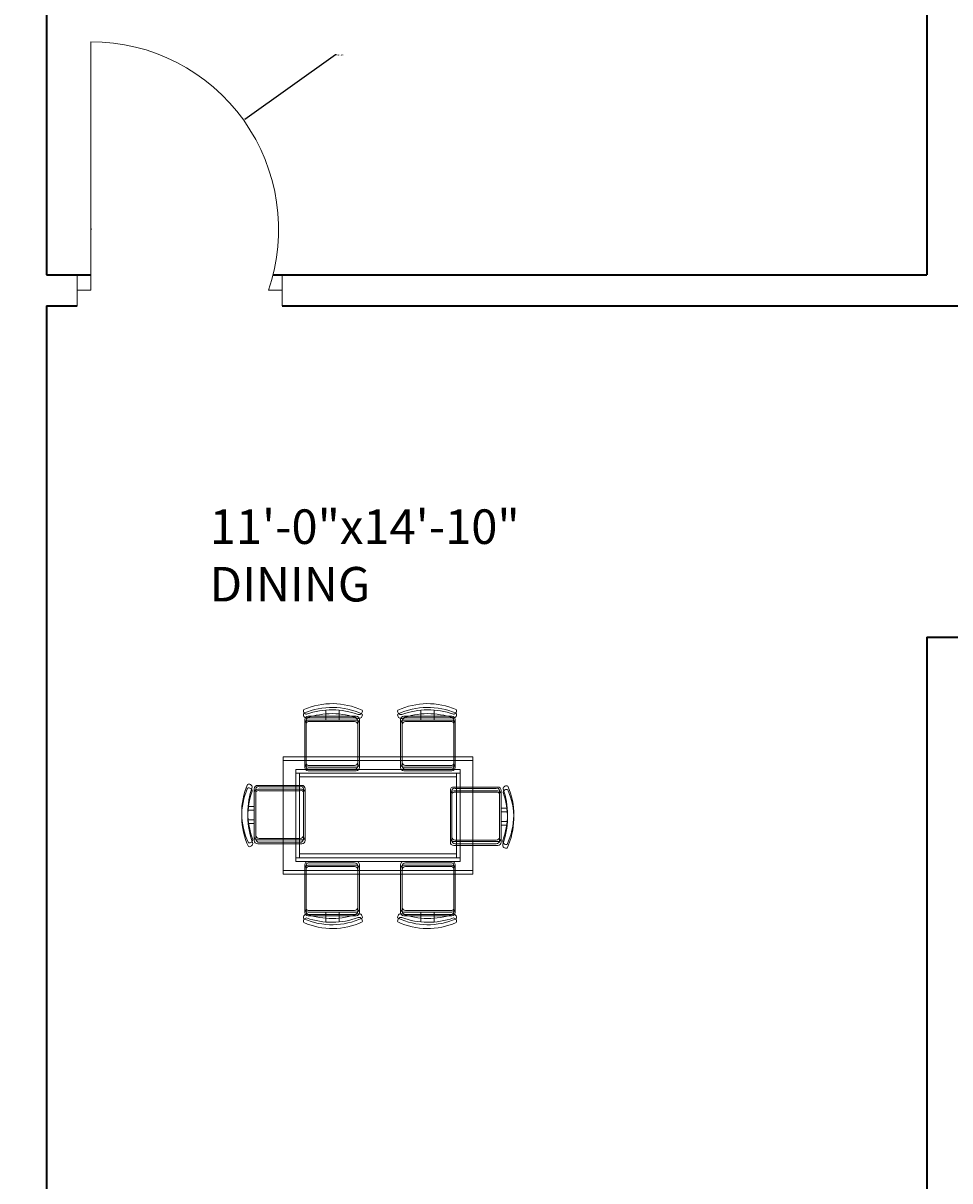
# Model space of a CAD drawing. Units: inches. Extents: x 2163 to 2982, y 1024 to 2288.
# Tile 20 of 22: x 2583 to 2718, y 1885 to 2053. Entities that reach past the tile are written whole.
import ezdxf

# ---------------------------------------------------------------- set-up
doc = ezdxf.new("R2010")
doc.units = ezdxf.units.IN
for name, color, linetype, lineweight in [('A-ANNO-DIMS', 2, 'Continuous', 18), ('A-AREA-IDEN', 7, 'Continuous', 18), ('A-DOOR', 11, 'Continuous', 18), ('A-FURN', 8, 'Continuous', 13), ('A-WALL', 7, 'Continuous', 35)]:
    doc.layers.add(name, color=color, linetype=linetype, lineweight=lineweight)
doc.styles.get("Standard").update_dxf_attribs({"font": 'arial.ttf'})
doc.dimstyles.get("Standard").update_dxf_attribs({"dimtxt": 0.18, "dimasz": 0.18, "dimexe": 0.18, "dimexo": 0.0625, "dimgap": 0.09, "dimtad": 0, "dimtih": 1, "dimtoh": 1, "dimdec": 4, "dimzin": 0, "dimdsep": 46, "dimtxsty": 'Standard', "dimcen": 0.09, "dimadec": 0, "dimazin": 0, "dimtfac": 1, "dimtdec": 4, "dimtofl": 0, "dimtmove": 0, "dimatfit": 3, "dimfxl": 1, "dimtolj": 1, "dimtzin": 0, "dimarcsym": 0})

# ---------------------------------------------------------------- blocks, each defined once
blk = doc.blocks.new('TABLE-DINING')
for points in [[(0, 17.02), (27.45, 17.02), (27.45, 0.55), (0, 0.55)], [(0, 17.02), (27.45, 17.02), (27.45, 0.55), (0, 0.55)], [(0, 17.02), (27.45, 17.02), (27.45, 0.55), (0, 0.55)], [(0, 17.02), (27.45, 17.02), (27.45, 0.55), (0, 0.55)], [(0, 16.47), (27.45, 16.47), (27.45, 0), (0, 0)], [(0, 16.47), (27.45, 16.47), (27.45, 0), (0, 0)], [(0, 16.47), (27.45, 16.47), (27.45, 0), (0, 0)], [(0, 16.47), (27.45, 16.47), (27.45, 0), (0, 0)], [(1.83, 15.19), (25.62, 15.19), (25.62, 2.38), (1.83, 2.38)], [(1.83, 15.19), (25.62, 15.19), (25.62, 2.38), (1.83, 2.38)], [(1.83, 15.19), (25.62, 15.19), (25.62, 2.38), (1.83, 2.38)], [(1.83, 15.19), (25.62, 15.19), (25.62, 2.38), (1.83, 2.38)], [(1.83, 14.64), (25.62, 14.64), (25.62, 1.83), (1.83, 1.83)], [(1.83, 14.64), (25.62, 14.64), (25.62, 1.83), (1.83, 1.83)], [(1.83, 14.64), (25.62, 14.64), (25.62, 1.83), (1.83, 1.83)], [(1.83, 14.64), (25.62, 14.64), (25.62, 1.83), (1.83, 1.83)], [(2.38, 14.64), (25.07, 14.64), (25.07, 2.93), (2.38, 2.93)], [(2.38, 14.64), (25.07, 14.64), (25.07, 2.93), (2.38, 2.93)], [(2.38, 14.64), (25.07, 14.64), (25.07, 2.93), (2.38, 2.93)], [(2.38, 14.64), (25.07, 14.64), (25.07, 2.93), (2.38, 2.93)], [(2.38, 14.09), (25.07, 14.09), (25.07, 2.38), (2.38, 2.38)], [(2.38, 14.09), (25.07, 14.09), (25.07, 2.38), (2.38, 2.38)], [(2.38, 14.09), (25.07, 14.09), (25.07, 2.38), (2.38, 2.38)], [(2.38, 14.09), (25.07, 14.09), (25.07, 2.38), (2.38, 2.38)]]:
    blk.add_lwpolyline(points, close=True)
blk = doc.blocks.new('*D29')
at = {"layer": 'A-ANNO-DIMS', "color": 0, "lineweight": -2, "transparency": 16777216}
for p, q in [((2285.34, 1738.83), (2285.34, 2288.1)), ((2285.52, 2287.92), (2576.05, 2287.92)), ((2867.16, 2287.92), (2576.63, 2287.92)), ((2867.34, 2229.33), (2867.34, 2288.1))]:
    blk.add_line(p, q, dxfattribs=at)
at = {"layer": 'A-ANNO-DIMS', "color": 0, "transparency": 16777216}
for points in [[(2285.52, 2287.95), (2285.52, 2287.89), (2285.34, 2287.92)], [(2867.16, 2287.95), (2867.16, 2287.89), (2867.34, 2287.92)]]:
    blk.add_solid(points, dxfattribs=at)
at = {"layer": 'Defpoints', "color": 0, "transparency": 16777216}
for p in [(2867.34, 2287.92), (2867.34, 2229.27), (2285.34, 1738.77)]:
    blk.add_point(p, dxfattribs=at)
at = {"layer": 'A-ANNO-DIMS', "color": 0, "transparency": 16777216, "insert": (2576.34, 2287.92), "char_height": 0.18, "attachment_point": 5}
blk.add_mtext('\\A1;582', dxfattribs=at)
blk = doc.blocks.new('*D47')
at = {"layer": 'A-ANNO-DIMS', "color": 0, "lineweight": -2, "transparency": 16777216}
for p, q in [((2628.67, 2048.1), (2615.54, 2038.74)), ((2628.85, 2048.1), (2628.67, 2048.1)), ((2593.2, 2022.85), (2593.38, 2022.85)), ((2593.29, 2022.76), (2593.29, 2022.94))]:
    blk.add_line(p, q, dxfattribs=at)
at = {"layer": 'A-ANNO-DIMS', "color": 0, "transparency": 16777216}
blk.add_solid([(2615.53, 2038.76), (2615.56, 2038.71), (2615.4, 2038.63)], dxfattribs=at)
at = {"layer": 'Defpoints', "color": 0, "transparency": 16777216}
for p in [(2615.4, 2038.63), (2593.29, 2022.85)]:
    blk.add_point(p, dxfattribs=at)
at = {"layer": 'A-ANNO-DIMS', "color": 0, "transparency": 16777216, "insert": (2629.4, 2048.1), "char_height": 0.18, "attachment_point": 5}
blk.add_mtext('\\A1;R27.165', dxfattribs=at)

msp = doc.modelspace()

# ---------------------------------------------------------------- linework, layer by layer
at = {"layer": 'A-DOOR'}
for p, q in [((2593.2852, 2014.0188), (2593.2852, 2050.0188)), ((2591.2852, 2016.2688), (2591.2852, 2011.7688)), ((2620.9736, 2016.2688), (2620.9736, 2011.7688)), ((2591.2852, 2011.7688), (2591.2852, 2014.0188)), ((2591.2852, 2014.0188), (2593.2852, 2014.0188)), ((2620.9736, 2014.0188), (2618.9736, 2014.0188)), ((2620.9736, 2011.7688), (2620.9736, 2014.0188))]:
    msp.add_line(p, q, dxfattribs=at)
msp.add_arc((2593.2852, 2022.8537), 27.1652, 341.020745, 90, dxfattribs=at)
at = {"layer": 'A-FURN'}
for points in [[(2624.5142, 1952.6105, -0.17580919), (2631.9896, 1952.5539, 0.57839206), (2632.556, 1953.1766, 0.21452438), (2624.1178, 1953.2899, 0.55201397), (2624.5142, 1952.6105, -0.06507904)], [(2624.5142, 1952.6105, -0.17580919), (2631.9896, 1952.5539, 0.57839206), (2632.556, 1953.1766, 0.21452438), (2624.1178, 1953.2899, 0.55201397), (2624.5142, 1952.6105, -0.06507904)], [(2624.5142, 1952.6103, -0.17580919), (2631.9896, 1952.5536, 0.57839206), (2632.556, 1953.1764, 0.21452438), (2624.1178, 1953.2896, 0.55201397), (2624.5142, 1952.6103, -0.06507904)], [(2624.5142, 1952.6103, -0.17580919), (2631.9896, 1952.5536, 0.57839206), (2632.556, 1953.1764, 0.21452438), (2624.1178, 1953.2896, 0.55201397), (2624.5142, 1952.6103, -0.06507904)], [(2624.5142, 1952.0616, -0.17580919), (2631.9896, 1952.005, 0.57839206), (2632.556, 1952.6277, 0.21452438), (2624.1178, 1952.741, 0.55201397), (2624.5142, 1952.0616, -0.06507904)], [(2624.5142, 1952.0616, -0.17580919), (2631.9896, 1952.005, 0.57839206), (2632.556, 1952.6277, 0.21452438), (2624.1178, 1952.741, 0.55201397), (2624.5142, 1952.0616, -0.06507904)], [(2624.5142, 1952.0613, -0.17580919), (2631.9896, 1952.0047, 0.57839206), (2632.556, 1952.6274, 0.21452438), (2624.1178, 1952.7407, 0.55201397), (2624.5142, 1952.0613, -0.06507904)], [(2624.5142, 1952.0613, -0.17580919), (2631.9896, 1952.0047, 0.57839206), (2632.556, 1952.6274, 0.21452438), (2624.1178, 1952.7407, 0.55201397), (2624.5142, 1952.0613, -0.06507904)], [(2638.283, 1952.5539, -0.57839206), (2637.7167, 1953.1766, -0.21452438), (2646.1548, 1953.2899, -0.55201397), (2645.7584, 1952.6105, 0.1758092), (2638.283, 1952.5539)], [(2638.283, 1952.5539, -0.57839206), (2637.7167, 1953.1766, -0.21452438), (2646.1548, 1953.2899, -0.55201397), (2645.7584, 1952.6105, 0.1758092), (2638.283, 1952.5539)], [(2638.283, 1952.5536, -0.57839206), (2637.7167, 1953.1764, -0.21452438), (2646.1549, 1953.2896, -0.55201397), (2645.7584, 1952.6103, 0.1758092), (2638.283, 1952.5536)], [(2638.283, 1952.5536, -0.57839206), (2637.7167, 1953.1764, -0.21452438), (2646.1549, 1953.2896, -0.55201397), (2645.7584, 1952.6103, 0.1758092), (2638.283, 1952.5536)], [(2638.283, 1952.005, -0.57839206), (2637.7167, 1952.6277, -0.21452438), (2646.1548, 1952.741, -0.55201397), (2645.7584, 1952.0616, 0.1758092), (2638.283, 1952.005)], [(2638.283, 1952.005, -0.57839206), (2637.7167, 1952.6277, -0.21452438), (2646.1548, 1952.741, -0.55201397), (2645.7584, 1952.0616, 0.1758092), (2638.283, 1952.005)], [(2638.283, 1952.0047, -0.57839206), (2637.7167, 1952.6274, -0.21452438), (2646.1549, 1952.7407, -0.55201397), (2645.7584, 1952.0613, 0.1758092), (2638.283, 1952.0047)], [(2638.283, 1952.0047, -0.57839206), (2637.7167, 1952.6274, -0.21452438), (2646.1549, 1952.7407, -0.55201397), (2645.7584, 1952.0613, 0.1758092), (2638.283, 1952.0047)], [(2631.6725, 1952.3105), (2624.7325, 1952.3105, 0.41421356), (2624.247, 1951.825), (2624.247, 1945.4438, 0.41421356), (2624.7325, 1944.9583), (2631.6725, 1944.9583, 0.41421356), (2632.158, 1945.4438), (2632.158, 1951.825, 0.41421356), (2631.6725, 1952.3105)], [(2631.6725, 1952.3105), (2624.7325, 1952.3105, 0.41421356), (2624.247, 1951.825), (2624.247, 1945.4438, 0.41421356), (2624.7325, 1944.9583), (2631.6725, 1944.9583, 0.41421356), (2632.158, 1945.4438), (2632.158, 1951.825, 0.41421356), (2631.6725, 1952.3105)], [(2631.6725, 1952.3102), (2624.7326, 1952.3102, 0.41421356), (2624.247, 1951.8247), (2624.247, 1945.4436, 0.41421356), (2624.7326, 1944.958), (2631.6725, 1944.958, 0.41421356), (2632.158, 1945.4436), (2632.158, 1951.8247, 0.41421356), (2631.6725, 1952.3102)], [(2631.6725, 1952.3102), (2624.7326, 1952.3102, 0.41421356), (2624.247, 1951.8247), (2624.247, 1945.4436, 0.41421356), (2624.7326, 1944.958), (2631.6725, 1944.958, 0.41421356), (2632.158, 1945.4436), (2632.158, 1951.8247, 0.41421356), (2631.6725, 1952.3102)], [(2629.2348, 1952.3105), (2629.2348, 1953.1882, -0.06475861)], [(2629.2348, 1952.3105), (2629.2348, 1953.1882, -0.06475861)], [(2629.2348, 1952.3102), (2629.2348, 1953.1879, -0.06475861)], [(2629.2348, 1952.3102), (2629.2348, 1953.1879, -0.06475861)], [(2629.2348, 1951.7616), (2629.2348, 1952.6393, -0.06475861)], [(2629.2348, 1951.7616), (2629.2348, 1952.6393, -0.06475861)], [(2629.2348, 1951.7613), (2629.2348, 1952.639, -0.06475861)], [(2629.2348, 1951.7613), (2629.2348, 1952.639, -0.06475861)], [(2645.5401, 1952.3105, -0.41421356), (2646.0256, 1951.825), (2646.0256, 1945.4438, -0.41421356), (2645.5401, 1944.9583), (2638.6001, 1944.9583, -0.41421356), (2638.1146, 1945.4438), (2638.1146, 1951.825, -0.41421356), (2638.6001, 1952.3105), (2645.5401, 1952.3105)], [(2645.5401, 1952.3105, -0.41421356), (2646.0256, 1951.825), (2646.0256, 1945.4438, -0.41421356), (2645.5401, 1944.9583), (2638.6001, 1944.9583, -0.41421356), (2638.1146, 1945.4438), (2638.1146, 1951.825, -0.41421356), (2638.6001, 1952.3105), (2645.5401, 1952.3105)], [(2645.5401, 1952.3102, -0.41421356), (2646.0256, 1951.8247), (2646.0256, 1945.4436, -0.41421356), (2645.5401, 1944.958), (2638.6002, 1944.958, -0.41421356), (2638.1146, 1945.4436), (2638.1146, 1951.8247, -0.41421356), (2638.6002, 1952.3102), (2645.5401, 1952.3102)], [(2645.5401, 1952.3102, -0.41421356), (2646.0256, 1951.8247), (2646.0256, 1945.4436, -0.41421356), (2645.5401, 1944.958), (2638.6002, 1944.958, -0.41421356), (2638.1146, 1945.4436), (2638.1146, 1951.8247, -0.41421356), (2638.6002, 1952.3102), (2645.5401, 1952.3102)], [(2641.0378, 1952.3105), (2641.0378, 1953.1882, 0.06475861)], [(2641.0378, 1952.3105), (2641.0378, 1953.1882, 0.06475861)], [(2641.0378, 1952.3102), (2641.0378, 1953.1879, 0.06475861)], [(2641.0378, 1952.3102), (2641.0378, 1953.1879, 0.06475861)], [(2641.0378, 1951.7616), (2641.0378, 1952.6393, 0.06475861)], [(2641.0378, 1951.7616), (2641.0378, 1952.6393, 0.06475861)], [(2641.0378, 1951.7613), (2641.0378, 1952.639, 0.06475861)], [(2641.0378, 1951.7613), (2641.0378, 1952.639, 0.06475861)], [(2631.6725, 1951.7616), (2624.7325, 1951.7616, 0.41421356), (2624.247, 1951.2761), (2624.247, 1944.8949, 0.41421356), (2624.7325, 1944.4094), (2631.6725, 1944.4094, 0.41421356), (2632.158, 1944.8949), (2632.158, 1951.2761, 0.41421356), (2631.6725, 1951.7616)], [(2631.6725, 1951.7616), (2624.7325, 1951.7616, 0.41421356), (2624.247, 1951.2761), (2624.247, 1944.8949, 0.41421356), (2624.7325, 1944.4094), (2631.6725, 1944.4094, 0.41421356), (2632.158, 1944.8949), (2632.158, 1951.2761, 0.41421356), (2631.6725, 1951.7616)], [(2631.6725, 1951.7613), (2624.7326, 1951.7613, 0.41421356), (2624.247, 1951.2758), (2624.247, 1944.8946, 0.41421356), (2624.7326, 1944.4091), (2631.6725, 1944.4091, 0.41421356), (2632.158, 1944.8946), (2632.158, 1951.2758, 0.41421356), (2631.6725, 1951.7613)], [(2631.6725, 1951.7613), (2624.7326, 1951.7613, 0.41421356), (2624.247, 1951.2758), (2624.247, 1944.8946, 0.41421356), (2624.7326, 1944.4091), (2631.6725, 1944.4091, 0.41421356), (2632.158, 1944.8946), (2632.158, 1951.2758, 0.41421356), (2631.6725, 1951.7613)], [(2645.5401, 1951.7616, -0.41421356), (2646.0256, 1951.2761), (2646.0256, 1944.8949, -0.41421356), (2645.5401, 1944.4094), (2638.6001, 1944.4094, -0.41421356), (2638.1146, 1944.8949), (2638.1146, 1951.2761, -0.41421356), (2638.6001, 1951.7616), (2645.5401, 1951.7616)], [(2645.5401, 1951.7616, -0.41421356), (2646.0256, 1951.2761), (2646.0256, 1944.8949, -0.41421356), (2645.5401, 1944.4094), (2638.6001, 1944.4094, -0.41421356), (2638.1146, 1944.8949), (2638.1146, 1951.2761, -0.41421356), (2638.6001, 1951.7616), (2645.5401, 1951.7616)], [(2645.5401, 1951.7613, -0.41421356), (2646.0256, 1951.2758), (2646.0256, 1944.8946, -0.41421356), (2645.5401, 1944.4091), (2638.6002, 1944.4091, -0.41421356), (2638.1146, 1944.8946), (2638.1146, 1951.2758, -0.41421356), (2638.6002, 1951.7613), (2645.5401, 1951.7613)], [(2645.5401, 1951.7613, -0.41421356), (2646.0256, 1951.2758), (2646.0256, 1944.8946, -0.41421356), (2645.5401, 1944.4091), (2638.6002, 1944.4091, -0.41421356), (2638.1146, 1944.8946), (2638.1146, 1951.2758, -0.41421356), (2638.6002, 1951.7613), (2645.5401, 1951.7613)], [(2616.6935, 1934.5585, -0.57839206), (2616.0707, 1933.9922, -0.21452438), (2615.9575, 1942.4304, -0.55201397), (2616.6368, 1942.0339, 0.17580937), (2616.6935, 1934.5585)], [(2616.6935, 1934.5585, -0.57839206), (2616.0707, 1933.9922, -0.21452438), (2615.9575, 1942.4304, -0.55201397), (2616.6368, 1942.0339, 0.17580937), (2616.6935, 1934.5585)], [(2616.6935, 1934.5582, -0.57839206), (2616.0708, 1933.9919, -0.21452438), (2615.9575, 1942.4301, -0.55201397), (2616.6369, 1942.0336, 0.17580937), (2616.6935, 1934.5582)], [(2616.6935, 1934.5582, -0.57839206), (2616.0708, 1933.9919, -0.21452438), (2615.9575, 1942.4301, -0.55201397), (2616.6369, 1942.0336, 0.17580937), (2616.6935, 1934.5582)], [(2616.6935, 1934.0096, -0.57839206), (2616.0707, 1933.4433, -0.21452438), (2615.9575, 1941.8814, -0.55201397), (2616.6368, 1941.485, 0.17580937), (2616.6935, 1934.0096)], [(2616.6935, 1934.0096, -0.57839206), (2616.0707, 1933.4433, -0.21452438), (2615.9575, 1941.8814, -0.55201397), (2616.6368, 1941.485, 0.17580937), (2616.6935, 1934.0096)], [(2616.6935, 1934.0093, -0.57839206), (2616.0708, 1933.443, -0.21452438), (2615.9575, 1941.8812, -0.55201397), (2616.6369, 1941.4847, 0.17580937), (2616.6935, 1934.0093)], [(2616.6935, 1934.0093, -0.57839206), (2616.0708, 1933.443, -0.21452438), (2615.9575, 1941.8812, -0.55201397), (2616.6369, 1941.4847, 0.17580937), (2616.6935, 1934.0093)], [(2616.9369, 1941.8156, -0.41421356), (2617.4224, 1942.3011), (2623.8035, 1942.3011, -0.41421356), (2624.2891, 1941.8156), (2624.2891, 1934.8756, -0.41421356), (2623.8035, 1934.3901), (2617.4224, 1934.3901, -0.41421356), (2616.9369, 1934.8756), (2616.9369, 1941.8156)], [(2616.9369, 1941.8156, -0.41421356), (2617.4224, 1942.3011), (2623.8035, 1942.3011, -0.41421356), (2624.2891, 1941.8156), (2624.2891, 1934.8756, -0.41421356), (2623.8035, 1934.3901), (2617.4224, 1934.3901, -0.41421356), (2616.9369, 1934.8756), (2616.9369, 1941.8156)], [(2616.9369, 1941.8153, -0.41421356), (2617.4224, 1942.3008), (2623.8036, 1942.3008, -0.41421356), (2624.2891, 1941.8153), (2624.2891, 1934.8754, -0.41421356), (2623.8036, 1934.3898), (2617.4224, 1934.3898, -0.41421356), (2616.9369, 1934.8754), (2616.9369, 1941.8153)], [(2616.9369, 1941.8153, -0.41421356), (2617.4224, 1942.3008), (2623.8036, 1942.3008, -0.41421356), (2624.2891, 1941.8153), (2624.2891, 1934.8754, -0.41421356), (2623.8036, 1934.3898), (2617.4224, 1934.3898, -0.41421356), (2616.9369, 1934.8754), (2616.9369, 1941.8153)], [(2652.6743, 1941.5779, 0.41421356), (2652.1888, 1942.0634), (2645.8077, 1942.0634, 0.41421356), (2645.3221, 1941.5779), (2645.3221, 1934.638, 0.41421356), (2645.8077, 1934.1524), (2652.1888, 1934.1524, 0.41421356), (2652.6743, 1934.638), (2652.6743, 1941.5779)], [(2652.6743, 1941.5779, 0.41421356), (2652.1888, 1942.0634), (2645.8077, 1942.0634, 0.41421356), (2645.3221, 1941.5779), (2645.3221, 1934.638, 0.41421356), (2645.8077, 1934.1524), (2652.1888, 1934.1524, 0.41421356), (2652.6743, 1934.638), (2652.6743, 1941.5779)], [(2652.6743, 1941.5776, 0.41421356), (2652.1888, 1942.0631), (2645.8077, 1942.0631, 0.41421356), (2645.3221, 1941.5776), (2645.3221, 1934.6377, 0.41421356), (2645.8077, 1934.1522), (2652.1888, 1934.1522, 0.41421356), (2652.6743, 1934.6377), (2652.6743, 1941.5776)], [(2652.6743, 1941.5776, 0.41421356), (2652.1888, 1942.0631), (2645.8077, 1942.0631, 0.41421356), (2645.3221, 1941.5776), (2645.3221, 1934.6377, 0.41421356), (2645.8077, 1934.1522), (2652.1888, 1934.1522, 0.41421356), (2652.6743, 1934.6377), (2652.6743, 1941.5776)], [(2652.9744, 1941.7962, -0.17580919), (2652.9178, 1934.3208, 0.57839206), (2653.5405, 1933.7545, 0.21452438), (2653.6537, 1942.1927, 0.55201397), (2652.9744, 1941.7963, -0.06507904)], [(2652.9744, 1941.7962, -0.17580919), (2652.9178, 1934.3208, 0.57839206), (2653.5405, 1933.7545, 0.21452438), (2653.6537, 1942.1927, 0.55201397), (2652.9744, 1941.7963, -0.06507904)], [(2652.9744, 1941.796, -0.17580919), (2652.9178, 1934.3205, 0.57839206), (2653.5405, 1933.7542, 0.21452438), (2653.6537, 1942.1924, 0.55201397), (2652.9744, 1941.796, -0.06507904)], [(2652.9744, 1941.796, -0.17580919), (2652.9178, 1934.3205, 0.57839206), (2653.5405, 1933.7542, 0.21452438), (2653.6537, 1942.1924, 0.55201397), (2652.9744, 1941.796, -0.06507904)], [(2616.9369, 1941.2667, -0.41421356), (2617.4224, 1941.7522), (2623.8035, 1941.7522, -0.41421356), (2624.2891, 1941.2667), (2624.2891, 1934.3267, -0.41421356), (2623.8035, 1933.8412), (2617.4224, 1933.8412, -0.41421356), (2616.9369, 1934.3267), (2616.9369, 1941.2667)], [(2616.9369, 1941.2667, -0.41421356), (2617.4224, 1941.7522), (2623.8035, 1941.7522, -0.41421356), (2624.2891, 1941.2667), (2624.2891, 1934.3267, -0.41421356), (2623.8035, 1933.8412), (2617.4224, 1933.8412, -0.41421356), (2616.9369, 1934.3267), (2616.9369, 1941.2667)], [(2616.9369, 1941.2664, -0.41421356), (2617.4224, 1941.7519), (2623.8036, 1941.7519, -0.41421356), (2624.2891, 1941.2664), (2624.2891, 1934.3264, -0.41421356), (2623.8036, 1933.8409), (2617.4224, 1933.8409, -0.41421356), (2616.9369, 1934.3264), (2616.9369, 1941.2664)], [(2616.9369, 1941.2664, -0.41421356), (2617.4224, 1941.7519), (2623.8036, 1941.7519, -0.41421356), (2624.2891, 1941.2664), (2624.2891, 1934.3264, -0.41421356), (2623.8036, 1933.8409), (2617.4224, 1933.8409, -0.41421356), (2616.9369, 1934.3264), (2616.9369, 1941.2664)], [(2652.6743, 1941.029, 0.41421356), (2652.1888, 1941.5145), (2645.8077, 1941.5145, 0.41421356), (2645.3221, 1941.029), (2645.3221, 1934.0891, 0.41421356), (2645.8077, 1933.6035), (2652.1888, 1933.6035, 0.41421356), (2652.6743, 1934.0891), (2652.6743, 1941.029)], [(2652.6743, 1941.029, 0.41421356), (2652.1888, 1941.5145), (2645.8077, 1941.5145, 0.41421356), (2645.3221, 1941.029), (2645.3221, 1934.0891, 0.41421356), (2645.8077, 1933.6035), (2652.1888, 1933.6035, 0.41421356), (2652.6743, 1934.0891), (2652.6743, 1941.029)], [(2652.6743, 1941.0287, 0.41421356), (2652.1888, 1941.5142), (2645.8077, 1941.5142, 0.41421356), (2645.3221, 1941.0287), (2645.3221, 1934.0888, 0.41421356), (2645.8077, 1933.6032), (2652.1888, 1933.6032, 0.41421356), (2652.6743, 1934.0888), (2652.6743, 1941.0287)], [(2652.6743, 1941.0287, 0.41421356), (2652.1888, 1941.5142), (2645.8077, 1941.5142, 0.41421356), (2645.3221, 1941.0287), (2645.3221, 1934.0888, 0.41421356), (2645.8077, 1933.6032), (2652.1888, 1933.6032, 0.41421356), (2652.6743, 1934.0888), (2652.6743, 1941.0287)], [(2652.9744, 1941.2473, -0.17580919), (2652.9178, 1933.7719, 0.57839206), (2653.5405, 1933.2056, 0.21452438), (2653.6537, 1941.6438, 0.55201397), (2652.9744, 1941.2473, -0.06507904)], [(2652.9744, 1941.2473, -0.17580919), (2652.9178, 1933.7719, 0.57839206), (2653.5405, 1933.2056, 0.21452438), (2653.6537, 1941.6438, 0.55201397), (2652.9744, 1941.2473, -0.06507904)], [(2652.9744, 1941.247, -0.17580919), (2652.9178, 1933.7716, 0.57839206), (2653.5405, 1933.2053, 0.21452438), (2653.6537, 1941.6435, 0.55201397), (2652.9744, 1941.247, -0.06507904)], [(2652.9744, 1941.247, -0.17580919), (2652.9178, 1933.7716, 0.57839206), (2653.5405, 1933.2053, 0.21452438), (2653.6537, 1941.6435, 0.55201397), (2652.9744, 1941.247, -0.06507904)], [(2616.9369, 1937.3133), (2616.0592, 1937.3133, 0.06475861)], [(2616.9369, 1937.3133), (2616.0592, 1937.3133, 0.06475861)], [(2616.9369, 1937.313), (2616.0592, 1937.313, 0.06475861)], [(2616.9369, 1937.313), (2616.0592, 1937.313, 0.06475861)], [(2616.9369, 1936.7644), (2616.0592, 1936.7644, 0.06475861)], [(2616.9369, 1936.7644), (2616.0592, 1936.7644, 0.06475861)], [(2616.9369, 1936.7641), (2616.0592, 1936.7641, 0.06475861)], [(2616.9369, 1936.7641), (2616.0592, 1936.7641, 0.06475861)], [(2652.6743, 1937.0756), (2653.552, 1937.0756, -0.06475861)], [(2652.6743, 1937.0756), (2653.552, 1937.0756, -0.06475861)], [(2652.6743, 1937.0753), (2653.552, 1937.0753, -0.06475861)], [(2652.6743, 1937.0753), (2653.552, 1937.0753, -0.06475861)], [(2652.6743, 1936.5267), (2653.552, 1936.5267, -0.06475861)], [(2652.6743, 1936.5267), (2653.552, 1936.5267, -0.06475861)], [(2652.6743, 1936.5264), (2653.552, 1936.5264, -0.06475861)], [(2652.6743, 1936.5264), (2653.552, 1936.5264, -0.06475861)], [(2631.6725, 1923.9448), (2624.7325, 1923.9448, -0.41421356), (2624.247, 1924.4303), (2624.247, 1930.8114, -0.41421356), (2624.7325, 1931.297), (2631.6725, 1931.297, -0.41421356), (2632.158, 1930.8114), (2632.158, 1924.4303, -0.41421356), (2631.6725, 1923.9448)], [(2631.6725, 1923.9448), (2624.7325, 1923.9448, -0.41421356), (2624.247, 1924.4303), (2624.247, 1930.8114, -0.41421356), (2624.7325, 1931.297), (2631.6725, 1931.297, -0.41421356), (2632.158, 1930.8114), (2632.158, 1924.4303, -0.41421356), (2631.6725, 1923.9448)], [(2631.6725, 1923.9445), (2624.7326, 1923.9445, -0.41421356), (2624.247, 1924.43), (2624.247, 1930.8111, -0.41421356), (2624.7326, 1931.2967), (2631.6725, 1931.2967, -0.41421356), (2632.158, 1930.8111), (2632.158, 1924.43, -0.41421356), (2631.6725, 1923.9445)], [(2631.6725, 1923.9445), (2624.7326, 1923.9445, -0.41421356), (2624.247, 1924.43), (2624.247, 1930.8111, -0.41421356), (2624.7326, 1931.2967), (2631.6725, 1931.2967, -0.41421356), (2632.158, 1930.8111), (2632.158, 1924.43, -0.41421356), (2631.6725, 1923.9445)], [(2631.6725, 1923.3958), (2624.7325, 1923.3958, -0.41421356), (2624.247, 1923.8814), (2624.247, 1930.2625, -0.41421356), (2624.7325, 1930.748), (2631.6725, 1930.748, -0.41421356), (2632.158, 1930.2625), (2632.158, 1923.8814, -0.41421356), (2631.6725, 1923.3958)], [(2631.6725, 1923.3958), (2624.7325, 1923.3958, -0.41421356), (2624.247, 1923.8814), (2624.247, 1930.2625, -0.41421356), (2624.7325, 1930.748), (2631.6725, 1930.748, -0.41421356), (2632.158, 1930.2625), (2632.158, 1923.8814, -0.41421356), (2631.6725, 1923.3958)], [(2631.6725, 1923.3956), (2624.7326, 1923.3956, -0.41421356), (2624.247, 1923.8811), (2624.247, 1930.2622, -0.41421356), (2624.7326, 1930.7478), (2631.6725, 1930.7478, -0.41421356), (2632.158, 1930.2622), (2632.158, 1923.8811, -0.41421356), (2631.6725, 1923.3956)], [(2631.6725, 1923.3956), (2624.7326, 1923.3956, -0.41421356), (2624.247, 1923.8811), (2624.247, 1930.2622, -0.41421356), (2624.7326, 1930.7478), (2631.6725, 1930.7478, -0.41421356), (2632.158, 1930.2622), (2632.158, 1923.8811, -0.41421356), (2631.6725, 1923.3956)], [(2645.5401, 1923.9448, 0.41421356), (2646.0256, 1924.4303), (2646.0256, 1930.8114, 0.41421356), (2645.5401, 1931.297), (2638.6001, 1931.297, 0.41421356), (2638.1146, 1930.8114), (2638.1146, 1924.4303, 0.41421356), (2638.6001, 1923.9448), (2645.5401, 1923.9448)], [(2645.5401, 1923.9448, 0.41421356), (2646.0256, 1924.4303), (2646.0256, 1930.8114, 0.41421356), (2645.5401, 1931.297), (2638.6001, 1931.297, 0.41421356), (2638.1146, 1930.8114), (2638.1146, 1924.4303, 0.41421356), (2638.6001, 1923.9448), (2645.5401, 1923.9448)], [(2645.5401, 1923.9445, 0.41421356), (2646.0256, 1924.43), (2646.0256, 1930.8111, 0.41421356), (2645.5401, 1931.2967), (2638.6002, 1931.2967, 0.41421356), (2638.1146, 1930.8111), (2638.1146, 1924.43, 0.41421356), (2638.6002, 1923.9445), (2645.5401, 1923.9445)], [(2645.5401, 1923.9445, 0.41421356), (2646.0256, 1924.43), (2646.0256, 1930.8111, 0.41421356), (2645.5401, 1931.2967), (2638.6002, 1931.2967, 0.41421356), (2638.1146, 1930.8111), (2638.1146, 1924.43, 0.41421356), (2638.6002, 1923.9445), (2645.5401, 1923.9445)], [(2645.5401, 1923.3958, 0.41421356), (2646.0256, 1923.8814), (2646.0256, 1930.2625, 0.41421356), (2645.5401, 1930.748), (2638.6001, 1930.748, 0.41421356), (2638.1146, 1930.2625), (2638.1146, 1923.8814, 0.41421356), (2638.6001, 1923.3958), (2645.5401, 1923.3958)], [(2645.5401, 1923.3958, 0.41421356), (2646.0256, 1923.8814), (2646.0256, 1930.2625, 0.41421356), (2645.5401, 1930.748), (2638.6001, 1930.748, 0.41421356), (2638.1146, 1930.2625), (2638.1146, 1923.8814, 0.41421356), (2638.6001, 1923.3958), (2645.5401, 1923.3958)], [(2645.5401, 1923.3956, 0.41421356), (2646.0256, 1923.8811), (2646.0256, 1930.2622, 0.41421356), (2645.5401, 1930.7478), (2638.6002, 1930.7478, 0.41421356), (2638.1146, 1930.2622), (2638.1146, 1923.8811, 0.41421356), (2638.6002, 1923.3956), (2645.5401, 1923.3956)], [(2645.5401, 1923.3956, 0.41421356), (2646.0256, 1923.8811), (2646.0256, 1930.2622, 0.41421356), (2645.5401, 1930.7478), (2638.6002, 1930.7478, 0.41421356), (2638.1146, 1930.2622), (2638.1146, 1923.8811, 0.41421356), (2638.6002, 1923.3956), (2645.5401, 1923.3956)], [(2631.9896, 1923.7013, -0.57839206), (2632.556, 1923.0786, -0.21452438), (2624.1178, 1922.9654, -0.55201397), (2624.5142, 1923.6447, 0.17580929), (2631.9896, 1923.7013)], [(2631.9896, 1923.7013, -0.57839206), (2632.556, 1923.0786, -0.21452438), (2624.1178, 1922.9654, -0.55201397), (2624.5142, 1923.6447, 0.17580929), (2631.9896, 1923.7013)], [(2631.9896, 1923.7011, -0.57839206), (2632.556, 1923.0783, -0.21452438), (2624.1178, 1922.9651, -0.55201397), (2624.5142, 1923.6444, 0.17580929), (2631.9896, 1923.7011)], [(2631.9896, 1923.7011, -0.57839206), (2632.556, 1923.0783, -0.21452438), (2624.1178, 1922.9651, -0.55201397), (2624.5142, 1923.6444, 0.17580929), (2631.9896, 1923.7011)], [(2629.2348, 1923.9448), (2629.2348, 1923.0671, 0.06475861)], [(2629.2348, 1923.9448), (2629.2348, 1923.0671, 0.06475861)], [(2629.2348, 1923.9445), (2629.2348, 1923.0668, 0.06475861)], [(2629.2348, 1923.9445), (2629.2348, 1923.0668, 0.06475861)], [(2629.2348, 1923.3958), (2629.2348, 1922.5182, 0.06475861)], [(2629.2348, 1923.3958), (2629.2348, 1922.5182, 0.06475861)], [(2629.2348, 1923.3956), (2629.2348, 1922.5179, 0.06475861)], [(2629.2348, 1923.3956), (2629.2348, 1922.5179, 0.06475861)], [(2645.7584, 1923.6447, -0.17580928), (2638.283, 1923.7013, 0.57839206), (2637.7167, 1923.0786, 0.21452438), (2646.1548, 1922.9654, 0.55201397), (2645.7584, 1923.6447, -0.06507904)], [(2645.7584, 1923.6447, -0.17580928), (2638.283, 1923.7013, 0.57839206), (2637.7167, 1923.0786, 0.21452438), (2646.1548, 1922.9654, 0.55201397), (2645.7584, 1923.6447, -0.06507904)], [(2645.7584, 1923.6444, -0.17580928), (2638.283, 1923.7011, 0.57839206), (2637.7167, 1923.0783, 0.21452438), (2646.1549, 1922.9651, 0.55201397), (2645.7584, 1923.6444, -0.06507904)], [(2645.7584, 1923.6444, -0.17580928), (2638.283, 1923.7011, 0.57839206), (2637.7167, 1923.0783, 0.21452438), (2646.1549, 1922.9651, 0.55201397), (2645.7584, 1923.6444, -0.06507904)], [(2641.0378, 1923.9448), (2641.0378, 1923.0671, -0.06475861)], [(2641.0378, 1923.9448), (2641.0378, 1923.0671, -0.06475861)], [(2641.0378, 1923.9445), (2641.0378, 1923.0668, -0.06475861)], [(2641.0378, 1923.9445), (2641.0378, 1923.0668, -0.06475861)], [(2641.0378, 1923.3958), (2641.0378, 1922.5182, -0.06475861)], [(2641.0378, 1923.3958), (2641.0378, 1922.5182, -0.06475861)], [(2641.0378, 1923.3956), (2641.0378, 1922.5179, -0.06475861)], [(2641.0378, 1923.3956), (2641.0378, 1922.5179, -0.06475861)], [(2631.9896, 1923.1524, -0.57839206), (2632.556, 1922.5297, -0.21452438), (2624.1178, 1922.4165, -0.55201397), (2624.5142, 1923.0958, 0.17580929), (2631.9896, 1923.1524)], [(2631.9896, 1923.1524, -0.57839206), (2632.556, 1922.5297, -0.21452438), (2624.1178, 1922.4165, -0.55201397), (2624.5142, 1923.0958, 0.17580929), (2631.9896, 1923.1524)], [(2631.9896, 1923.1521, -0.57839206), (2632.556, 1922.5294, -0.21452438), (2624.1178, 1922.4162, -0.55201397), (2624.5142, 1923.0955, 0.17580929), (2631.9896, 1923.1521)], [(2631.9896, 1923.1521, -0.57839206), (2632.556, 1922.5294, -0.21452438), (2624.1178, 1922.4162, -0.55201397), (2624.5142, 1923.0955, 0.17580929), (2631.9896, 1923.1521)], [(2645.7584, 1923.0958, -0.17580928), (2638.283, 1923.1524, 0.57839206), (2637.7167, 1922.5297, 0.21452438), (2646.1548, 1922.4165, 0.55201397), (2645.7584, 1923.0958, -0.06507904)], [(2645.7584, 1923.0958, -0.17580928), (2638.283, 1923.1524, 0.57839206), (2637.7167, 1922.5297, 0.21452438), (2646.1548, 1922.4165, 0.55201397), (2645.7584, 1923.0958, -0.06507904)], [(2645.7584, 1923.0955, -0.17580928), (2638.283, 1923.1521, 0.57839206), (2637.7167, 1922.5294, 0.21452438), (2646.1549, 1922.4162, 0.55201397), (2645.7584, 1923.0955, -0.06507904)], [(2645.7584, 1923.0955, -0.17580928), (2638.283, 1923.1521, 0.57839206), (2637.7167, 1922.5294, 0.21452438), (2646.1549, 1922.4162, 0.55201397), (2645.7584, 1923.0955, -0.06507904)]]:
    msp.add_lwpolyline(points, format="xyb", dxfattribs=at)
for points in [[(2624.7355, 1952.0918), (2631.4537, 1952.0918, -0.41421356), (2631.9393, 1951.6063), (2631.9393, 1945.6626, -0.41421356), (2631.4537, 1945.177), (2624.7355, 1945.177, -0.51206948), (2624.4657, 1945.6626), (2624.4657, 1951.6063, -0.51206948)], [(2624.7355, 1952.0918), (2631.4537, 1952.0918, -0.41421356), (2631.9393, 1951.6063), (2631.9393, 1945.6626, -0.41421356), (2631.4537, 1945.177), (2624.7355, 1945.177, -0.51206948), (2624.4657, 1945.6626), (2624.4657, 1951.6063, -0.51206948)], [(2624.7355, 1952.0915), (2631.4538, 1952.0915, -0.41421356), (2631.9393, 1951.606), (2631.9393, 1945.6623, -0.41421356), (2631.4538, 1945.1768), (2624.7355, 1945.1768, -0.51206948), (2624.4658, 1945.6623), (2624.4658, 1951.606, -0.51206948)], [(2624.7355, 1952.0915), (2631.4538, 1952.0915, -0.41421356), (2631.9393, 1951.606), (2631.9393, 1945.6623, -0.41421356), (2631.4538, 1945.1768), (2624.7355, 1945.1768, -0.51206948), (2624.4658, 1945.6623), (2624.4658, 1951.606, -0.51206948)], [(2645.5371, 1952.0918), (2638.8189, 1952.0918, 0.41421356), (2638.3333, 1951.6063), (2638.3333, 1945.6626, 0.41421356), (2638.8189, 1945.177), (2645.5371, 1945.177, 0.51206948), (2645.8069, 1945.6626), (2645.8069, 1951.6063, 0.51206948)], [(2645.5371, 1952.0918), (2638.8189, 1952.0918, 0.41421356), (2638.3333, 1951.6063), (2638.3333, 1945.6626, 0.41421356), (2638.8189, 1945.177), (2645.5371, 1945.177, 0.51206948), (2645.8069, 1945.6626), (2645.8069, 1951.6063, 0.51206948)], [(2645.5371, 1952.0915), (2638.8189, 1952.0915, 0.41421356), (2638.3334, 1951.606), (2638.3334, 1945.6623, 0.41421356), (2638.8189, 1945.1768), (2645.5371, 1945.1768, 0.51206948), (2645.8069, 1945.6623), (2645.8069, 1951.606, 0.51206948)], [(2645.5371, 1952.0915), (2638.8189, 1952.0915, 0.41421356), (2638.3334, 1951.606), (2638.3334, 1945.6623, 0.41421356), (2638.8189, 1945.1768), (2645.5371, 1945.1768, 0.51206948), (2645.8069, 1945.6623), (2645.8069, 1951.606, 0.51206948)], [(2624.7355, 1951.5429), (2631.4537, 1951.5429, -0.41421356), (2631.9393, 1951.0573), (2631.9393, 1945.1137, -0.41421356), (2631.4537, 1944.6281), (2624.7355, 1944.6281, -0.51206948), (2624.4657, 1945.1137), (2624.4657, 1951.0573, -0.51206948)], [(2624.7355, 1951.5429), (2631.4537, 1951.5429, -0.41421356), (2631.9393, 1951.0573), (2631.9393, 1945.1137, -0.41421356), (2631.4537, 1944.6281), (2624.7355, 1944.6281, -0.51206948), (2624.4657, 1945.1137), (2624.4657, 1951.0573, -0.51206948)], [(2624.7355, 1951.5426), (2631.4538, 1951.5426, -0.41421356), (2631.9393, 1951.057), (2631.9393, 1945.1134, -0.41421356), (2631.4538, 1944.6278), (2624.7355, 1944.6278, -0.51206948), (2624.4658, 1945.1134), (2624.4658, 1951.057, -0.51206948)], [(2624.7355, 1951.5426), (2631.4538, 1951.5426, -0.41421356), (2631.9393, 1951.057), (2631.9393, 1945.1134, -0.41421356), (2631.4538, 1944.6278), (2624.7355, 1944.6278, -0.51206948), (2624.4658, 1945.1134), (2624.4658, 1951.057, -0.51206948)], [(2645.5371, 1951.5429), (2638.8189, 1951.5429, 0.41421356), (2638.3333, 1951.0573), (2638.3333, 1945.1137, 0.41421356), (2638.8189, 1944.6281), (2645.5371, 1944.6281, 0.51206948), (2645.8069, 1945.1137), (2645.8069, 1951.0573, 0.51206948)], [(2645.5371, 1951.5429), (2638.8189, 1951.5429, 0.41421356), (2638.3333, 1951.0573), (2638.3333, 1945.1137, 0.41421356), (2638.8189, 1944.6281), (2645.5371, 1944.6281, 0.51206948), (2645.8069, 1945.1137), (2645.8069, 1951.0573, 0.51206948)], [(2645.5371, 1951.5426), (2638.8189, 1951.5426, 0.41421356), (2638.3334, 1951.057), (2638.3334, 1945.1134, 0.41421356), (2638.8189, 1944.6278), (2645.5371, 1944.6278, 0.51206948), (2645.8069, 1945.1134), (2645.8069, 1951.057, 0.51206948)], [(2645.5371, 1951.5426), (2638.8189, 1951.5426, 0.41421356), (2638.3334, 1951.057), (2638.3334, 1945.1134, 0.41421356), (2638.8189, 1944.6278), (2645.5371, 1944.6278, 0.51206948), (2645.8069, 1945.1134), (2645.8069, 1951.057, 0.51206948)], [(2617.1556, 1941.8126), (2617.1556, 1935.0944, 0.41421356), (2617.6411, 1934.6089), (2623.5848, 1934.6089, 0.41421356), (2624.0703, 1935.0944), (2624.0703, 1941.8126, 0.51206948), (2623.5848, 1942.0824), (2617.6411, 1942.0824, 0.51206948)], [(2617.1556, 1941.8126), (2617.1556, 1935.0944, 0.41421356), (2617.6411, 1934.6089), (2623.5848, 1934.6089, 0.41421356), (2624.0703, 1935.0944), (2624.0703, 1941.8126, 0.51206948), (2623.5848, 1942.0824), (2617.6411, 1942.0824, 0.51206948)], [(2617.1556, 1941.8124), (2617.1556, 1935.0941, 0.41421356), (2617.6411, 1934.6086), (2623.5848, 1934.6086, 0.41421356), (2624.0703, 1935.0941), (2624.0703, 1941.8124, 0.51206948), (2623.5848, 1942.0821), (2617.6411, 1942.0821, 0.51206948)], [(2617.1556, 1941.8124), (2617.1556, 1935.0941, 0.41421356), (2617.6411, 1934.6086), (2623.5848, 1934.6086, 0.41421356), (2624.0703, 1935.0941), (2624.0703, 1941.8124, 0.51206948), (2623.5848, 1942.0821), (2617.6411, 1942.0821, 0.51206948)], [(2652.4556, 1941.575), (2652.4556, 1934.8567, -0.41421356), (2651.9701, 1934.3712), (2646.0264, 1934.3712, -0.41421356), (2645.5409, 1934.8567), (2645.5409, 1941.575, -0.51206948), (2646.0264, 1941.8447), (2651.9701, 1941.8447, -0.51206948)], [(2652.4556, 1941.575), (2652.4556, 1934.8567, -0.41421356), (2651.9701, 1934.3712), (2646.0264, 1934.3712, -0.41421356), (2645.5409, 1934.8567), (2645.5409, 1941.575, -0.51206948), (2646.0264, 1941.8447), (2651.9701, 1941.8447, -0.51206948)], [(2652.4556, 1941.5747), (2652.4556, 1934.8564, -0.41421356), (2651.9701, 1934.3709), (2646.0264, 1934.3709, -0.41421356), (2645.5409, 1934.8564), (2645.5409, 1941.5747, -0.51206948), (2646.0264, 1941.8444), (2651.9701, 1941.8444, -0.51206948)], [(2652.4556, 1941.5747), (2652.4556, 1934.8564, -0.41421356), (2651.9701, 1934.3709), (2646.0264, 1934.3709, -0.41421356), (2645.5409, 1934.8564), (2645.5409, 1941.5747, -0.51206948), (2646.0264, 1941.8444), (2651.9701, 1941.8444, -0.51206948)], [(2617.1556, 1941.2637), (2617.1556, 1934.5455, 0.41421356), (2617.6411, 1934.0599), (2623.5848, 1934.0599, 0.41421356), (2624.0703, 1934.5455), (2624.0703, 1941.2637, 0.51206948), (2623.5848, 1941.5335), (2617.6411, 1941.5335, 0.51206948)], [(2617.1556, 1941.2637), (2617.1556, 1934.5455, 0.41421356), (2617.6411, 1934.0599), (2623.5848, 1934.0599, 0.41421356), (2624.0703, 1934.5455), (2624.0703, 1941.2637, 0.51206948), (2623.5848, 1941.5335), (2617.6411, 1941.5335, 0.51206948)], [(2617.1556, 1941.2634), (2617.1556, 1934.5452, 0.41421356), (2617.6411, 1934.0596), (2623.5848, 1934.0596, 0.41421356), (2624.0703, 1934.5452), (2624.0703, 1941.2634, 0.51206948), (2623.5848, 1941.5332), (2617.6411, 1941.5332, 0.51206948)], [(2617.1556, 1941.2634), (2617.1556, 1934.5452, 0.41421356), (2617.6411, 1934.0596), (2623.5848, 1934.0596, 0.41421356), (2624.0703, 1934.5452), (2624.0703, 1941.2634, 0.51206948), (2623.5848, 1941.5332), (2617.6411, 1941.5332, 0.51206948)], [(2652.4556, 1941.026), (2652.4556, 1934.3078, -0.41421356), (2651.9701, 1933.8223), (2646.0264, 1933.8223, -0.41421356), (2645.5409, 1934.3078), (2645.5409, 1941.026, -0.51206948), (2646.0264, 1941.2958), (2651.9701, 1941.2958, -0.51206948)], [(2652.4556, 1941.026), (2652.4556, 1934.3078, -0.41421356), (2651.9701, 1933.8223), (2646.0264, 1933.8223, -0.41421356), (2645.5409, 1934.3078), (2645.5409, 1941.026, -0.51206948), (2646.0264, 1941.2958), (2651.9701, 1941.2958, -0.51206948)], [(2652.4556, 1941.0258), (2652.4556, 1934.3075, -0.41421356), (2651.9701, 1933.822), (2646.0264, 1933.822, -0.41421356), (2645.5409, 1934.3075), (2645.5409, 1941.0258, -0.51206948), (2646.0264, 1941.2955), (2651.9701, 1941.2955, -0.51206948)], [(2652.4556, 1941.0258), (2652.4556, 1934.3075, -0.41421356), (2651.9701, 1933.822), (2646.0264, 1933.822, -0.41421356), (2645.5409, 1934.3075), (2645.5409, 1941.0258, -0.51206948), (2646.0264, 1941.2955), (2651.9701, 1941.2955, -0.51206948)], [(2624.7355, 1924.1635), (2631.4537, 1924.1635, 0.41421356), (2631.9393, 1924.649), (2631.9393, 1930.5927, 0.41421356), (2631.4537, 1931.0782), (2624.7355, 1931.0782, 0.51206948), (2624.4657, 1930.5927), (2624.4657, 1924.649, 0.51206948)], [(2624.7355, 1924.1635), (2631.4537, 1924.1635, 0.41421356), (2631.9393, 1924.649), (2631.9393, 1930.5927, 0.41421356), (2631.4537, 1931.0782), (2624.7355, 1931.0782, 0.51206948), (2624.4657, 1930.5927), (2624.4657, 1924.649, 0.51206948)], [(2624.7355, 1924.1632), (2631.4538, 1924.1632, 0.41421356), (2631.9393, 1924.6487), (2631.9393, 1930.5924, 0.41421356), (2631.4538, 1931.0779), (2624.7355, 1931.0779, 0.51206948), (2624.4658, 1930.5924), (2624.4658, 1924.6487, 0.51206948)], [(2624.7355, 1924.1632), (2631.4538, 1924.1632, 0.41421356), (2631.9393, 1924.6487), (2631.9393, 1930.5924, 0.41421356), (2631.4538, 1931.0779), (2624.7355, 1931.0779, 0.51206948), (2624.4658, 1930.5924), (2624.4658, 1924.6487, 0.51206948)], [(2624.7355, 1923.6146), (2631.4537, 1923.6146, 0.41421356), (2631.9393, 1924.1001), (2631.9393, 1930.0438, 0.41421356), (2631.4537, 1930.5293), (2624.7355, 1930.5293, 0.51206948), (2624.4657, 1930.0438), (2624.4657, 1924.1001, 0.51206948)], [(2624.7355, 1923.6146), (2631.4537, 1923.6146, 0.41421356), (2631.9393, 1924.1001), (2631.9393, 1930.0438, 0.41421356), (2631.4537, 1930.5293), (2624.7355, 1930.5293, 0.51206948), (2624.4657, 1930.0438), (2624.4657, 1924.1001, 0.51206948)], [(2624.7355, 1923.6143), (2631.4538, 1923.6143, 0.41421356), (2631.9393, 1924.0998), (2631.9393, 1930.0435, 0.41421356), (2631.4538, 1930.529), (2624.7355, 1930.529, 0.51206948), (2624.4658, 1930.0435), (2624.4658, 1924.0998, 0.51206948)], [(2624.7355, 1923.6143), (2631.4538, 1923.6143, 0.41421356), (2631.9393, 1924.0998), (2631.9393, 1930.0435, 0.41421356), (2631.4538, 1930.529), (2624.7355, 1930.529, 0.51206948), (2624.4658, 1930.0435), (2624.4658, 1924.0998, 0.51206948)], [(2645.5371, 1924.1635), (2638.8189, 1924.1635, -0.41421356), (2638.3333, 1924.649), (2638.3333, 1930.5927, -0.41421356), (2638.8189, 1931.0782), (2645.5371, 1931.0782, -0.51206948), (2645.8069, 1930.5927), (2645.8069, 1924.649, -0.51206948)], [(2645.5371, 1924.1635), (2638.8189, 1924.1635, -0.41421356), (2638.3333, 1924.649), (2638.3333, 1930.5927, -0.41421356), (2638.8189, 1931.0782), (2645.5371, 1931.0782, -0.51206948), (2645.8069, 1930.5927), (2645.8069, 1924.649, -0.51206948)], [(2645.5371, 1923.6146), (2638.8189, 1923.6146, -0.41421356), (2638.3333, 1924.1001), (2638.3333, 1930.0438, -0.41421356), (2638.8189, 1930.5293), (2645.5371, 1930.5293, -0.51206948), (2645.8069, 1930.0438), (2645.8069, 1924.1001, -0.51206948)], [(2645.5371, 1923.6146), (2638.8189, 1923.6146, -0.41421356), (2638.3333, 1924.1001), (2638.3333, 1930.0438, -0.41421356), (2638.8189, 1930.5293), (2645.5371, 1930.5293, -0.51206948), (2645.8069, 1930.0438), (2645.8069, 1924.1001, -0.51206948)], [(2645.5371, 1924.1632), (2638.8189, 1924.1632, -0.41421356), (2638.3334, 1924.6487), (2638.3334, 1930.5924, -0.41421356), (2638.8189, 1931.0779), (2645.5371, 1931.0779, -0.51206948), (2645.8069, 1930.5924), (2645.8069, 1924.6487, -0.51206948)], [(2645.5371, 1924.1632), (2638.8189, 1924.1632, -0.41421356), (2638.3334, 1924.6487), (2638.3334, 1930.5924, -0.41421356), (2638.8189, 1931.0779), (2645.5371, 1931.0779, -0.51206948), (2645.8069, 1930.5924), (2645.8069, 1924.6487, -0.51206948)], [(2645.5371, 1923.6143), (2638.8189, 1923.6143, -0.41421356), (2638.3334, 1924.0998), (2638.3334, 1930.0435, -0.41421356), (2638.8189, 1930.529), (2645.5371, 1930.529, -0.51206948), (2645.8069, 1930.0435), (2645.8069, 1924.0998, -0.51206948)], [(2645.5371, 1923.6143), (2638.8189, 1923.6143, -0.41421356), (2638.3334, 1924.0998), (2638.3334, 1930.0435, -0.41421356), (2638.8189, 1930.529), (2645.5371, 1930.529, -0.51206948), (2645.8069, 1930.0435), (2645.8069, 1924.0998, -0.51206948)]]:
    msp.add_lwpolyline(points, format="xyb", close=True, dxfattribs=at)
for points in [[(2627.2922, 1953.2042), (2627.2922, 1952.3105)], [(2627.2922, 1953.2042), (2627.2922, 1952.3105)], [(2627.2922, 1953.2039), (2627.2922, 1952.3102)], [(2627.2922, 1953.2039), (2627.2922, 1952.3102)], [(2627.2922, 1952.6552), (2627.2922, 1951.7616)], [(2627.2922, 1952.6552), (2627.2922, 1951.7616)], [(2627.2922, 1952.6549), (2627.2922, 1951.7613)], [(2627.2922, 1952.6549), (2627.2922, 1951.7613)], [(2642.9804, 1953.2042), (2642.9804, 1952.3105)], [(2642.9804, 1953.2042), (2642.9804, 1952.3105)], [(2642.9804, 1953.2039), (2642.9804, 1952.3102)], [(2642.9804, 1953.2039), (2642.9804, 1952.3102)], [(2642.9804, 1952.6552), (2642.9804, 1951.7616)], [(2642.9804, 1952.6552), (2642.9804, 1951.7616)], [(2642.9804, 1952.6549), (2642.9804, 1951.7613)], [(2642.9804, 1952.6549), (2642.9804, 1951.7613)], [(2616.0432, 1939.2559), (2616.9369, 1939.2559)], [(2616.0432, 1939.2559), (2616.9369, 1939.2559)], [(2616.0432, 1939.2556), (2616.9369, 1939.2556)], [(2616.0432, 1939.2556), (2616.9369, 1939.2556)], [(2616.0432, 1938.707), (2616.9369, 1938.707)], [(2616.0432, 1938.707), (2616.9369, 1938.707)], [(2616.0432, 1938.7067), (2616.9369, 1938.7067)], [(2616.0432, 1938.7067), (2616.9369, 1938.7067)], [(2653.568, 1939.0182), (2652.6743, 1939.0182)], [(2653.568, 1939.0182), (2652.6743, 1939.0182)], [(2653.568, 1939.0179), (2652.6743, 1939.0179)], [(2653.568, 1939.0179), (2652.6743, 1939.0179)], [(2653.568, 1938.4693), (2652.6743, 1938.4693)], [(2653.568, 1938.4693), (2652.6743, 1938.4693)], [(2653.568, 1938.469), (2652.6743, 1938.469)], [(2653.568, 1938.469), (2652.6743, 1938.469)], [(2627.2922, 1923.0511), (2627.2922, 1923.9448)], [(2627.2922, 1923.0511), (2627.2922, 1923.9448)], [(2627.2922, 1923.0508), (2627.2922, 1923.9445)], [(2627.2922, 1923.0508), (2627.2922, 1923.9445)], [(2627.2922, 1922.5022), (2627.2922, 1923.3958)], [(2627.2922, 1922.5022), (2627.2922, 1923.3958)], [(2627.2922, 1922.5019), (2627.2922, 1923.3956)], [(2627.2922, 1922.5019), (2627.2922, 1923.3956)], [(2642.9804, 1923.0511), (2642.9804, 1923.9448)], [(2642.9804, 1923.0511), (2642.9804, 1923.9448)], [(2642.9804, 1923.0508), (2642.9804, 1923.9445)], [(2642.9804, 1923.0508), (2642.9804, 1923.9445)], [(2642.9804, 1922.5022), (2642.9804, 1923.3958)], [(2642.9804, 1922.5022), (2642.9804, 1923.3958)], [(2642.9804, 1922.5019), (2642.9804, 1923.3956)], [(2642.9804, 1922.5019), (2642.9804, 1923.3956)]]:
    msp.add_lwpolyline(points, dxfattribs=at)
at = {"layer": 'A-WALL'}
for p, q in [((2586.8389, 2172.2688), (2586.8389, 2016.2688)), ((2714.3389, 2172.2688), (2714.3389, 2016.2688)), ((2586.8389, 2016.2688), (2593.2852, 2016.2688)), ((2619.6402, 2016.2688), (2714.3389, 2016.2688)), ((2586.8389, 2011.7688), (2591.2852, 2011.7688)), ((2586.8389, 2011.7688), (2586.8389, 1719.2751)), ((2620.9736, 2011.7688), (2718.8389, 2011.7688)), ((2714.3389, 1963.7688), (2720.5891, 1963.7688)), ((2714.3389, 1963.7688), (2714.3389, 1882.7688))]:
    msp.add_line(p, q, dxfattribs=at)

# ---------------------------------------------------------------- block references
at = {"layer": 'A-FURN'}
msp.add_blockref('TABLE-DINING', (2621.1199, 1929.433), dxfattribs=at)

# ---------------------------------------------------------------- texts
at = {"layer": 'A-AREA-IDEN', "insert": (2610.4807, 1982.2713), "char_height": 5, "attachment_point": 1}
msp.add_mtext_dynamic_manual_height_columns('11\'-0"x14\'-10"\\PDINING', width=89.902194, gutter_width=12.5, heights=[0], dxfattribs=at)

# ---------------------------------------------------------------- dimensions: what is measured, and where the dimension line sits
at = {"layer": 'A-ANNO-DIMS'}
dim = msp.add_linear_dim(base=(2867.3389, 2287.9188), p1=(2285.3389, 1738.7688), p2=(2867.3389, 2229.2688), dimstyle='Standard', override={"dimdec": 0, "dimlfac": 1, "dimrnd": 0, "dimzin": 0, "dimdsep": 46, "dimlunit": 2}, dxfattribs=at)
dim.commit()
dim.dimension.update_dxf_attribs({"geometry": '*D29', "text_midpoint": (2576.3389, 2287.9188)})
dim = msp.add_radius_dim(center=(2593.2852, 2022.8537), mpoint=(2615.3978, 2038.6328), dimstyle='Standard', override={"dimdec": 3, "dimlfac": 1, "dimrnd": 0, "dimzin": 0, "dimdsep": 46, "dimlunit": 2}, dxfattribs=at)
dim.commit()
dim.dimension.update_dxf_attribs({"geometry": '*D47', "text_midpoint": (2629.3957, 2048.1003), "dimtype": 164})

doc.saveas('drawing.dxf')
